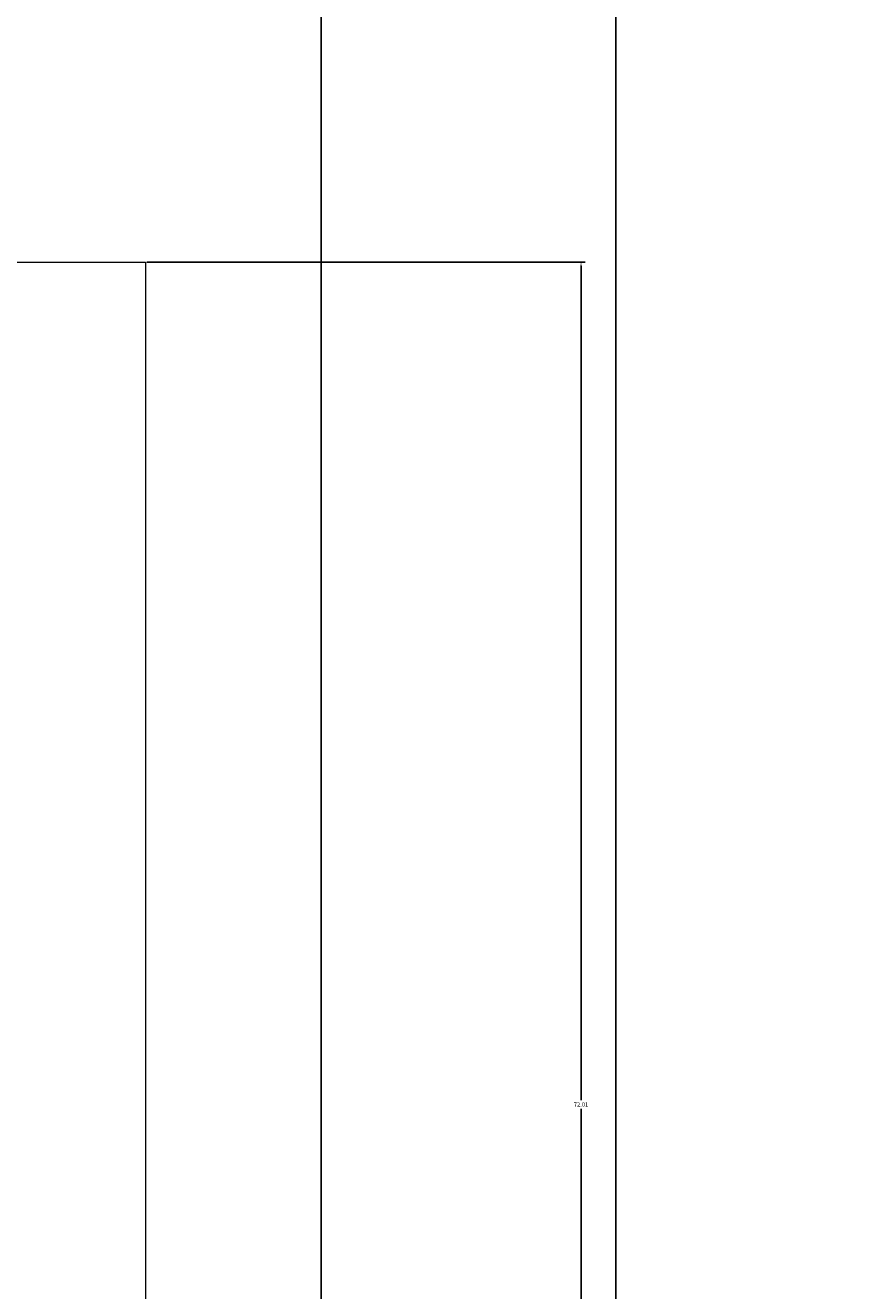
# Model space of a CAD drawing. Units: inches. Extents: x 2231 to 2461, y 2045 to 2455.
# Tile 48 of 95: x 2336 to 2371, y 2217 to 2271. Entities that reach past the tile are written whole.
import ezdxf

# ---------------------------------------------------------------- set-up
doc = ezdxf.new("R2010")
doc.units = ezdxf.units.IN
doc.layers.add('A-ANNO-DIMS', color=2, linetype='Continuous', lineweight=18)
doc.layers.add('A-FURN', color=9, linetype='Continuous', lineweight=18)
doc.styles.get("Standard").update_dxf_attribs({"font": 'arial.ttf'})
doc.dimstyles.get("Standard").update_dxf_attribs({"dimtxt": 0.18, "dimasz": 0.18, "dimexe": 0.18, "dimexo": 0.0625, "dimgap": 0.09, "dimtad": 0, "dimtih": 1, "dimtoh": 1, "dimdec": 4, "dimzin": 0, "dimdsep": 46, "dimtxsty": 'Standard', "dimcen": 0.09, "dimadec": 0, "dimazin": 0, "dimtfac": 1, "dimtdec": 4, "dimtofl": 0, "dimtmove": 0, "dimatfit": 3, "dimfxl": 1, "dimtolj": 1, "dimtzin": 0, "dimarcsym": 0})

# ---------------------------------------------------------------- blocks, each defined once
blk = doc.blocks.new('*D52')
at = {"layer": 'A-ANNO-DIMS', "color": 0, "lineweight": -2, "transparency": 16777216}
for p, q in [((2330.794, 2306.77), (2330.794, 2044.803)), ((2360.794, 2306.77), (2360.794, 2044.803)), ((2330.974, 2044.983), (2345.575, 2044.983)), ((2360.614, 2044.983), (2346.012, 2044.983))]:
    blk.add_line(p, q, dxfattribs=at)
at = {"layer": 'A-ANNO-DIMS', "color": 0, "transparency": 16777216}
for points in [[(2330.974, 2045.013), (2330.974, 2044.953), (2330.794, 2044.983)], [(2360.614, 2045.013), (2360.614, 2044.953), (2360.794, 2044.983)]]:
    blk.add_solid(points, dxfattribs=at)
at = {"layer": 'Defpoints', "color": 0, "transparency": 16777216}
for p in [(2330.794, 2306.833), (2360.794, 2306.833), (2360.794, 2044.983)]:
    blk.add_point(p, dxfattribs=at)
at = {"layer": 'A-ANNO-DIMS', "color": 0, "transparency": 16777216, "insert": (2345.794, 2044.983), "char_height": 0.18, "attachment_point": 5}
blk.add_mtext('\\A1;30', dxfattribs=at)
blk = doc.blocks.new('*D64')
at = {"layer": 'A-ANNO-DIMS', "color": 0, "lineweight": -2, "transparency": 16777216}
for p, q in [((2340.73, 2261.358), (2359.48, 2261.358)), ((2359.3, 2261.178), (2359.3, 2225.535)), ((2359.3, 2189.528), (2359.3, 2225.171)), ((2340.73, 2189.348), (2359.48, 2189.348))]:
    blk.add_line(p, q, dxfattribs=at)
at = {"layer": 'A-ANNO-DIMS', "color": 0, "transparency": 16777216}
for points in [[(2359.27, 2261.178), (2359.33, 2261.178), (2359.3, 2261.358)], [(2359.27, 2189.528), (2359.33, 2189.528), (2359.3, 2189.348)]]:
    blk.add_solid(points, dxfattribs=at)
at = {"layer": 'Defpoints', "color": 0, "transparency": 16777216}
for p in [(2340.667, 2261.358), (2340.667, 2189.348), (2359.3, 2189.348)]:
    blk.add_point(p, dxfattribs=at)
at = {"layer": 'A-ANNO-DIMS', "color": 0, "transparency": 16777216, "insert": (2359.3, 2225.353), "char_height": 0.18, "attachment_point": 5}
blk.add_mtext('\\A1;72.01', dxfattribs=at)
blk = doc.blocks.new('*D66')
at = {"layer": 'A-ANNO-DIMS', "color": 0, "lineweight": -2, "transparency": 16777216}
for p, q in [((2348.189, 2096.895), (2348.189, 2454.645)), ((2348.369, 2454.465), (2378.167, 2454.465)), ((2408.614, 2454.465), (2378.815, 2454.465)), ((2408.794, 2096.895), (2408.794, 2454.645))]:
    blk.add_line(p, q, dxfattribs=at)
at = {"layer": 'A-ANNO-DIMS', "color": 0, "transparency": 16777216}
for points in [[(2348.369, 2454.495), (2348.369, 2454.435), (2348.189, 2454.465)], [(2408.614, 2454.495), (2408.614, 2454.435), (2408.794, 2454.465)]]:
    blk.add_solid(points, dxfattribs=at)
at = {"layer": 'Defpoints', "color": 0, "transparency": 16777216}
for p in [(2408.794, 2454.465), (2348.189, 2096.833), (2408.794, 2096.833)]:
    blk.add_point(p, dxfattribs=at)
at = {"layer": 'A-ANNO-DIMS', "color": 0, "transparency": 16777216, "insert": (2378.491, 2454.465), "char_height": 0.18, "attachment_point": 5}
blk.add_mtext('\\A1;60.6', dxfattribs=at)

msp = doc.modelspace()

# ---------------------------------------------------------------- linework, layer by layer
at = {"layer": 'A-FURN'}
msp.add_lwpolyline([(2285.6353, 2255.1137), (2285.6353, 2261.3584), (2340.6673, 2261.3584), (2340.6673, 2189.3477), (2285.6353, 2189.3477), (2285.6353, 2195.1137)], dxfattribs=at)

# ---------------------------------------------------------------- dimensions: what is measured, and where the dimension line sits
at = {"layer": 'A-ANNO-DIMS'}
for base, p1, p2, override, picture, middle in [((2408.7935, 2454.4653), (2348.1888, 2096.8328), (2408.7935, 2096.8328), {"dimdec": 1, "dimlfac": 1, "dimrnd": 0, "dimzin": 0, "dimdsep": 46, "dimlunit": 2}, '*D66', (2378.4912, 2454.4653)), ((2360.7935, 2044.9825), (2330.7935, 2306.8328), (2360.7935, 2306.8328), {"dimdec": 0, "dimlfac": 1, "dimrnd": 0, "dimzin": 0, "dimdsep": 46, "dimlunit": 2}, '*D52', (2345.7935, 2044.9825))]:
    dim = msp.add_linear_dim(base=base, p1=p1, p2=p2, dimstyle='Standard', override=override, dxfattribs=at)
    dim.commit()
    dim.dimension.update_dxf_attribs({"geometry": picture, "text_midpoint": middle})
dim = msp.add_linear_dim(base=(2359.2998, 2189.3477), p1=(2340.6673, 2261.3584), p2=(2340.6673, 2189.3477), angle=270, dimstyle='Standard', override={"dimdec": 2, "dimlfac": 1, "dimrnd": 0, "dimzin": 0, "dimdsep": 46, "dimlunit": 2}, dxfattribs=at)
dim.commit()
dim.dimension.update_dxf_attribs({"geometry": '*D64', "text_midpoint": (2359.2998, 2225.353)})

doc.saveas('drawing.dxf')
